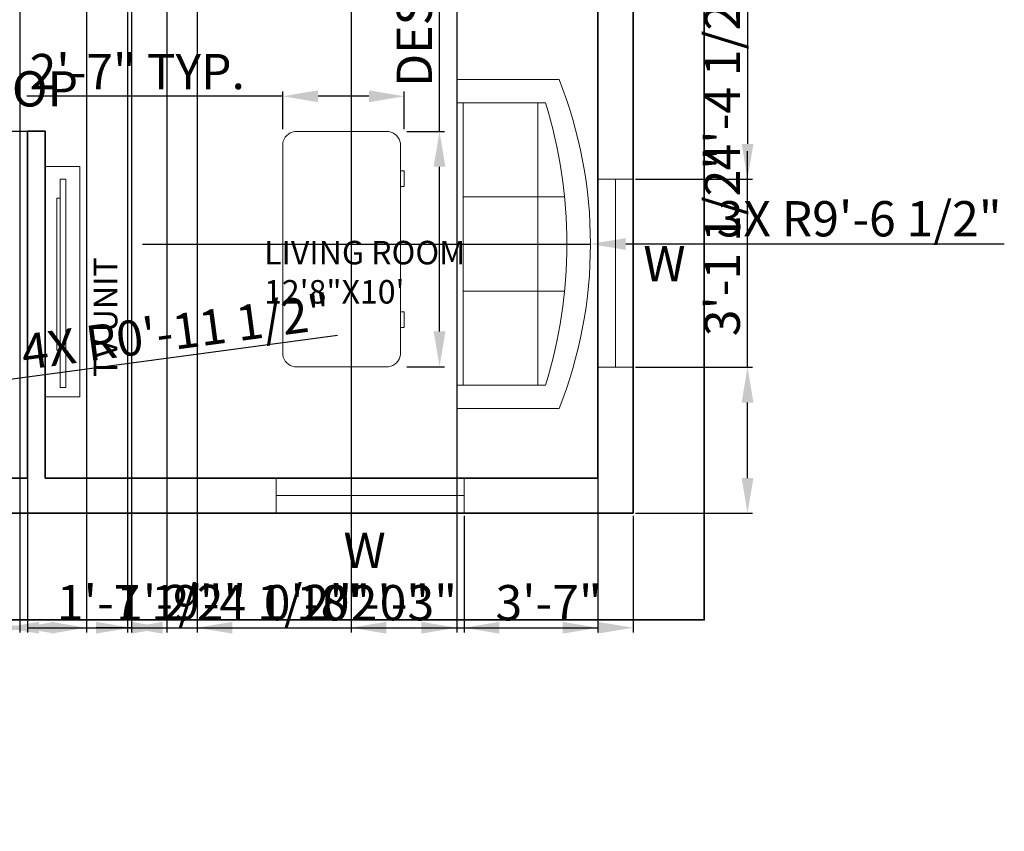
# Model space of a CAD drawing. Units: inches. Extents: x 53076 to 53578, y 41072 to 41816.
# Tile 2 of 4: x 53326 to 53578, y 41072 to 41279. Entities that reach past the tile are written whole.
import ezdxf

# ---------------------------------------------------------------- set-up
doc = ezdxf.new("R2010")
doc.units = ezdxf.units.IN
for name, color, linetype, lineweight in [('A-ANNO-DIMS', 2, 'Continuous', 18), ('A-ANNO-TEXT', 7, 'Continuous', 18), ('A-ANNO-TTLB', 7, 'Continuous', 35), ('A-AREA-IDEN', 7, 'Continuous', 18), ('A-DOOR', 3, 'Continuous', 25), ('A-EQPM', 8, 'Continuous', 18), ('A-FLOR-CASE', 9, 'Continuous', 18), ('A-FURN', 8, 'Continuous', 18), ('A-GLAZ', 4, 'Continuous', 18), ('A-WALL', 7, 'Continuous', 35)]:
    doc.layers.add(name, color=color, linetype=linetype, lineweight=lineweight)
doc.styles.get("Standard").update_dxf_attribs({"font": 'arial.ttf'})
doc.dimstyles.new('ISO-25', dxfattribs={"dimtxt": 9, "dimasz": 9, "dimexe": 1.25, "dimexo": 0.625, "dimtad": 1, "dimdec": 1, "dimrnd": 9, "dimlunit": 3, "dimtxsty": 'Standard', "dimcen": 2.5, "dimadec": 0, "dimazin": 0, "dimtfac": 1, "dimtdec": 1, "dimtmove": 0, "dimatfit": 3, "dimfxl": 1, "dimarcsym": 0})

# ---------------------------------------------------------------- blocks, each defined once
blk = doc.blocks.new('Sofa - Roundback 7 ft.')
for p, q in [((-12.00002, -32.4421), (-12.00003, -6.5971)), ((11.99997, -32.4421), (11.99998, -6.5971)), ((-36.000027, -34), (-36.000027, -11.4696)), ((35.99998, -34), (35.99998, -11.4696)), ((-35.999844, -13.3819), (35.9998, -13.3819)), ((-36.000027, -32.4421), (35.99998, -32.4421))]:
    blk.add_line(p, q)
for points in [[(-36.000027, -34), (-42.000027, -34), (-42.000027, -8)], [(41.99998, -8), (41.99998, -34), (35.99998, -34)]]:
    blk.add_lwpolyline(points)
for centre, radius, start, end in [((0, -114.25), 114.25, 68.43141, 111.5686), ((-0.00001, -127.1968), 121.1968, 72.72033, 107.2797)]:
    blk.add_arc(centre, radius, start, end)
blk = doc.blocks.new('Desk - 30 x 60 in.')
for p, q in [((-26.999995, 0), (26.999995, 0)), ((-29.999995, -27), (-29.999995, -3)), ((29.999995, -3), (29.999995, -27)), ((26.999995, -30), (-26.999995, -30)), ((-20.000005, -30), (-20.000005, -31)), ((-16.000005, -31), (-16.000005, -30)), ((15.999995, -31), (15.999995, -30)), ((19.999995, -30), (19.999995, -31)), ((-20.000005, -31), (-16.000005, -31)), ((19.999995, -31), (15.999995, -31))]:
    blk.add_line(p, q)
for centre, start, end in [((-26.499995, -3.5), 98.1301, 171.8699), ((26.499995, -3.5), 8.130102, 81.8699), ((-26.499995, -26.5), 188.1301, 261.8699), ((26.499995, -26.5), 278.1301, 351.8699)]:
    blk.add_arc(centre, 3.535534, start, end)
blk = doc.blocks.new('WIN-48IN')
for p, q in [((0, 48), (9, 48)), ((4.5, 48), (4.5, 0)), ((0, 0), (9, 0))]:
    blk.add_line(p, q)
blk = doc.blocks.new('*D28')
at = {"layer": 'A-ANNO-DIMS', "color": 0, "lineweight": -2, "transparency": 16777216}
for p, q in [((53433.43, 41250.06), (53433.43, 41352.45)), ((53425.06, 41250.06), (53434.68, 41250.06)), ((53433.43, 41199.06), (53433.43, 41241.06)), ((53425.06, 41190.06), (53434.68, 41190.06))]:
    blk.add_line(p, q, dxfattribs=at)
at = {"layer": 'A-ANNO-DIMS', "color": 0, "transparency": 16777216}
for points in [[(53431.93, 41241.06), (53434.93, 41241.06), (53433.43, 41250.06)], [(53431.93, 41199.06), (53434.93, 41199.06), (53433.43, 41190.06)]]:
    blk.add_solid(points, dxfattribs=at)
at = {"layer": 'Defpoints', "color": 0, "transparency": 16777216}
for p in [(53424.43, 41250.06), (53433.43, 41250.06), (53424.43, 41190.06)]:
    blk.add_point(p, dxfattribs=at)
at = {"layer": 'A-ANNO-DIMS', "color": 0, "transparency": 16777216, "insert": (53428.16, 41305.75), "char_height": 9, "attachment_point": 5, "rotation": 90}
blk.add_mtext('DESK 5\'-0" TYP.', dxfattribs=at)
blk = doc.blocks.new('*D29')
at = {"layer": 'A-ANNO-DIMS', "color": 0, "lineweight": -2, "transparency": 16777216}
for p, q in [((53393.43, 41250.68), (53393.43, 41260.31)), ((53424.43, 41250.68), (53424.43, 41260.31)), ((53393.43, 41259.06), (53328.17, 41259.06)), ((53415.43, 41259.06), (53402.43, 41259.06))]:
    blk.add_line(p, q, dxfattribs=at)
at = {"layer": 'A-ANNO-DIMS', "color": 0, "transparency": 16777216}
for points in [[(53402.43, 41260.56), (53402.43, 41257.56), (53393.43, 41259.06)], [(53415.43, 41260.56), (53415.43, 41257.56), (53424.43, 41259.06)]]:
    blk.add_solid(points, dxfattribs=at)
at = {"layer": 'Defpoints', "color": 0, "transparency": 16777216}
for p in [(53393.43, 41259.06), (53393.43, 41250.06), (53424.43, 41250.06)]:
    blk.add_point(p, dxfattribs=at)
at = {"layer": 'A-ANNO-DIMS', "color": 0, "transparency": 16777216, "insert": (53356.3, 41264.2), "char_height": 9, "attachment_point": 5}
blk.add_mtext('2\'-7" TYP.', dxfattribs=at)
blk = doc.blocks.new('*D30')
at = {"layer": 'A-ANNO-DIMS', "color": 0, "lineweight": -2, "transparency": 16777216}
for p, q in [((53312.97, 41194.48), (53318.55, 41194.48)), ((53317.3, 41185.48), (53317.3, 41170.44)), ((53312.97, 41161.44), (53318.55, 41161.44)), ((53317.3, 41161.44), (53317.3, 41071.52))]:
    blk.add_line(p, q, dxfattribs=at)
at = {"layer": 'A-ANNO-DIMS', "color": 0, "transparency": 16777216}
for points in [[(53315.8, 41185.48), (53318.8, 41185.48), (53317.3, 41194.48)], [(53315.8, 41170.44), (53318.8, 41170.44), (53317.3, 41161.44)]]:
    blk.add_solid(points, dxfattribs=at)
at = {"layer": 'Defpoints', "color": 0, "transparency": 16777216}
for p in [(53312.34, 41194.48), (53312.34, 41161.44), (53317.3, 41161.44)]:
    blk.add_point(p, dxfattribs=at)
at = {"layer": 'A-ANNO-DIMS', "color": 0, "transparency": 16777216, "insert": (53312.02, 41111.98), "char_height": 9, "attachment_point": 5, "rotation": 90}
blk.add_mtext('WC 2\'-9" TYP.', dxfattribs=at)
blk = doc.blocks.new('*D34')
at = {"layer": 'A-ANNO-DIMS', "color": 0, "lineweight": -2, "transparency": 16777216}
for p, q in [((53353.81, 41379.03), (53353.81, 41122.21)), ((53473.81, 41379.03), (53473.81, 41122.21)), ((53362.81, 41123.46), (53464.81, 41123.46))]:
    blk.add_line(p, q, dxfattribs=at)
at = {"layer": 'A-ANNO-DIMS', "color": 0, "transparency": 16777216}
for points in [[(53362.81, 41124.96), (53362.81, 41121.96), (53353.81, 41123.46)], [(53464.81, 41124.96), (53464.81, 41121.96), (53473.81, 41123.46)]]:
    blk.add_solid(points, dxfattribs=at)
at = {"layer": 'Defpoints', "color": 0, "transparency": 16777216}
for p in [(53353.81, 41379.66), (53473.81, 41379.66), (53473.81, 41123.46)]:
    blk.add_point(p, dxfattribs=at)
at = {"layer": 'A-ANNO-DIMS', "color": 0, "transparency": 16777216, "insert": (53413.81, 41128.68), "char_height": 9, "attachment_point": 5}
blk.add_mtext('10\'-0"', dxfattribs=at)
blk = doc.blocks.new('*D35')
at = {"layer": 'A-ANNO-DIMS', "color": 0, "lineweight": -2, "transparency": 16777216}
for p, q in [((53483.43, 41290.66), (53513.26, 41290.66)), ((53512.01, 41281.66), (53512.01, 41246.92)), ((53483.43, 41237.92), (53513.26, 41237.92))]:
    blk.add_line(p, q, dxfattribs=at)
at = {"layer": 'A-ANNO-DIMS', "color": 0, "transparency": 16777216}
for points in [[(53510.51, 41281.66), (53513.51, 41281.66), (53512.01, 41290.66)], [(53510.51, 41246.92), (53513.51, 41246.92), (53512.01, 41237.92)]]:
    blk.add_solid(points, dxfattribs=at)
at = {"layer": 'Defpoints', "color": 0, "transparency": 16777216}
for p in [(53482.81, 41290.66), (53482.81, 41237.92), (53512.01, 41237.92)]:
    blk.add_point(p, dxfattribs=at)
at = {"layer": 'A-ANNO-DIMS', "color": 0, "transparency": 16777216, "insert": (53506.73, 41264.29), "char_height": 9, "attachment_point": 5, "rotation": 90}
blk.add_mtext('4\'-4 1/2"', dxfattribs=at)
blk = doc.blocks.new('*D37')
at = {"layer": 'A-ANNO-DIMS', "color": 0, "lineweight": -2, "transparency": 16777216}
for p, q in [((53326.31, 41520.3), (53326.31, 41122.21)), ((53354.81, 41520.3), (53354.81, 41122.21)), ((53335.31, 41123.46), (53345.81, 41123.46)), ((53354.81, 41123.46), (53410.11, 41123.46))]:
    blk.add_line(p, q, dxfattribs=at)
at = {"layer": 'A-ANNO-DIMS', "color": 0, "transparency": 16777216}
for points in [[(53335.31, 41124.96), (53335.31, 41121.96), (53326.31, 41123.46)], [(53345.81, 41124.96), (53345.81, 41121.96), (53354.81, 41123.46)]]:
    blk.add_solid(points, dxfattribs=at)
at = {"layer": 'Defpoints', "color": 0, "transparency": 16777216}
for p in [(53326.31, 41520.92), (53354.81, 41520.92), (53354.81, 41123.46)]:
    blk.add_point(p, dxfattribs=at)
at = {"layer": 'A-ANNO-DIMS', "color": 0, "transparency": 16777216, "insert": (53386.96, 41128.73), "char_height": 9, "attachment_point": 5}
blk.add_mtext('2\'-4 1/2"', dxfattribs=at)
blk = doc.blocks.new('*D44')
at = {"layer": 'A-ANNO-DIMS', "color": 0, "lineweight": -2, "transparency": 16777216}
for p, q in [((53439.72, 41152.03), (53439.72, 41122.21)), ((53482.81, 41152.03), (53482.81, 41122.21)), ((53448.72, 41123.46), (53473.81, 41123.46))]:
    blk.add_line(p, q, dxfattribs=at)
at = {"layer": 'A-ANNO-DIMS', "color": 0, "transparency": 16777216}
for points in [[(53448.72, 41124.96), (53448.72, 41121.96), (53439.72, 41123.46)], [(53473.81, 41124.96), (53473.81, 41121.96), (53482.81, 41123.46)]]:
    blk.add_solid(points, dxfattribs=at)
at = {"layer": 'Defpoints', "color": 0, "transparency": 16777216}
for p in [(53439.72, 41152.66), (53482.81, 41152.66), (53482.81, 41123.46)]:
    blk.add_point(p, dxfattribs=at)
at = {"layer": 'A-ANNO-DIMS', "color": 0, "transparency": 16777216, "insert": (53461.27, 41128.68), "char_height": 9, "attachment_point": 5}
blk.add_mtext('3\'-7"', dxfattribs=at)
blk = doc.blocks.new('*D49')
at = {"layer": 'A-ANNO-DIMS', "color": 0, "lineweight": -2, "transparency": 16777216}
for p, q in [((53512.01, 41189.92), (53512.01, 41245.06)), ((53483.43, 41189.92), (53513.26, 41189.92)), ((53512.01, 41161.66), (53512.01, 41180.92)), ((53483.43, 41152.66), (53513.26, 41152.66))]:
    blk.add_line(p, q, dxfattribs=at)
at = {"layer": 'A-ANNO-DIMS', "color": 0, "transparency": 16777216}
for points in [[(53510.51, 41180.92), (53513.51, 41180.92), (53512.01, 41189.92)], [(53510.51, 41161.66), (53513.51, 41161.66), (53512.01, 41152.66)]]:
    blk.add_solid(points, dxfattribs=at)
at = {"layer": 'Defpoints', "color": 0, "transparency": 16777216}
for p in [(53482.81, 41189.92), (53512.01, 41189.92), (53482.81, 41152.66)]:
    blk.add_point(p, dxfattribs=at)
at = {"layer": 'A-ANNO-DIMS', "color": 0, "transparency": 16777216, "insert": (53506.72, 41221.99), "char_height": 9, "attachment_point": 5, "rotation": 90}
blk.add_mtext('3\'-1 1/2"', dxfattribs=at)
blk = doc.blocks.new('*D55')
at = {"layer": 'A-ANNO-DIMS', "color": 0, "lineweight": -2, "transparency": 16777216}
for p, q in [((53322.2, 41589.03), (53322.2, 41122.21)), ((53343.31, 41584.53), (53343.31, 41122.21)), ((53331.2, 41123.46), (53334.31, 41123.46)), ((53343.31, 41123.46), (53376.63, 41123.46))]:
    blk.add_line(p, q, dxfattribs=at)
at = {"layer": 'A-ANNO-DIMS', "color": 0, "transparency": 16777216}
for points in [[(53331.2, 41124.96), (53331.2, 41121.96), (53322.2, 41123.46)], [(53334.31, 41124.96), (53334.31, 41121.96), (53343.31, 41123.46)]]:
    blk.add_solid(points, dxfattribs=at)
at = {"layer": 'Defpoints', "color": 0, "transparency": 16777216}
for p in [(53322.2, 41589.66), (53343.31, 41585.16), (53343.31, 41123.46)]:
    blk.add_point(p, dxfattribs=at)
at = {"layer": 'A-ANNO-DIMS', "color": 0, "transparency": 16777216, "insert": (53364.47, 41128.68), "char_height": 9, "attachment_point": 5}
blk.add_mtext('1\'-9"', dxfattribs=at)
blk = doc.blocks.new('*D64')
at = {"layer": 'A-ANNO-DIMS', "color": 0, "lineweight": -2, "transparency": 16777216}
for p, q in [((53363.81, 41456.53), (53363.81, 41122.21)), ((53371.57, 41456.53), (53371.57, 41122.21)), ((53354.81, 41123.46), (53345.81, 41123.46)), ((53363.81, 41123.46), (53371.57, 41123.46)), ((53380.57, 41123.46), (53414.74, 41123.46))]:
    blk.add_line(p, q, dxfattribs=at)
at = {"layer": 'A-ANNO-DIMS', "color": 0, "transparency": 16777216}
for points in [[(53354.81, 41124.96), (53354.81, 41121.96), (53363.81, 41123.46)], [(53380.57, 41124.96), (53380.57, 41121.96), (53371.57, 41123.46)]]:
    blk.add_solid(points, dxfattribs=at)
at = {"layer": 'Defpoints', "color": 0, "transparency": 16777216}
for p in [(53363.81, 41457.16), (53371.57, 41457.16), (53371.57, 41123.46)]:
    blk.add_point(p, dxfattribs=at)
at = {"layer": 'A-ANNO-DIMS', "color": 0, "transparency": 16777216, "insert": (53402.15, 41128.68), "char_height": 9, "attachment_point": 5}
blk.add_mtext('0\'-8"', dxfattribs=at)
blk = doc.blocks.new('*D65')
at = {"layer": 'A-ANNO-DIMS', "color": 0, "lineweight": -2, "transparency": 16777216}
for p, q in [((53410.86, 41483.76), (53410.86, 41122.21)), ((53437.81, 41456.53), (53437.81, 41122.21)), ((53419.86, 41123.46), (53428.81, 41123.46))]:
    blk.add_line(p, q, dxfattribs=at)
at = {"layer": 'A-ANNO-DIMS', "color": 0, "transparency": 16777216}
for points in [[(53419.86, 41124.96), (53419.86, 41121.96), (53410.86, 41123.46)], [(53428.81, 41124.96), (53428.81, 41121.96), (53437.81, 41123.46)]]:
    blk.add_solid(points, dxfattribs=at)
at = {"layer": 'Defpoints', "color": 0, "transparency": 16777216}
for p in [(53410.86, 41484.39), (53437.81, 41457.16), (53437.81, 41123.46)]:
    blk.add_point(p, dxfattribs=at)
at = {"layer": 'A-ANNO-DIMS', "color": 0, "transparency": 16777216, "insert": (53424.33, 41128.68), "char_height": 9, "attachment_point": 5}
blk.add_mtext('2\'-3"', dxfattribs=at)
blk = doc.blocks.new('*D68')
at = {"layer": 'A-ANNO-DIMS', "color": 0, "lineweight": -2, "transparency": 16777216}
for p, q in [((53155.81, 41273.53), (53155.81, 41122.21)), ((53326.31, 41273.53), (53326.31, 41122.21)), ((53164.81, 41123.46), (53317.31, 41123.46))]:
    blk.add_line(p, q, dxfattribs=at)
at = {"layer": 'A-ANNO-DIMS', "color": 0, "transparency": 16777216}
for points in [[(53164.81, 41124.96), (53164.81, 41121.96), (53155.81, 41123.46)], [(53317.31, 41124.96), (53317.31, 41121.96), (53326.31, 41123.46)]]:
    blk.add_solid(points, dxfattribs=at)
at = {"layer": 'Defpoints', "color": 0, "transparency": 16777216}
for p in [(53155.81, 41274.16), (53326.31, 41274.16), (53326.31, 41123.46)]:
    blk.add_point(p, dxfattribs=at)
at = {"layer": 'A-ANNO-DIMS', "color": 0, "transparency": 16777216, "insert": (53241.06, 41128.73), "char_height": 9, "attachment_point": 5}
blk.add_mtext('14\'-2 1/2"', dxfattribs=at)
blk = doc.blocks.new('*D69')
at = {"layer": 'A-ANNO-DIMS', "color": 0, "lineweight": -2, "transparency": 16777216}
for p, q in [((53328.31, 41249.53), (53328.31, 41122.21)), ((53308.69, 41245.03), (53308.69, 41122.21)), ((53317.69, 41123.46), (53319.31, 41123.46)), ((53328.31, 41123.46), (53382.6, 41123.46))]:
    blk.add_line(p, q, dxfattribs=at)
at = {"layer": 'A-ANNO-DIMS', "color": 0, "transparency": 16777216}
for points in [[(53317.69, 41124.96), (53317.69, 41121.96), (53308.69, 41123.46)], [(53319.31, 41124.96), (53319.31, 41121.96), (53328.31, 41123.46)]]:
    blk.add_solid(points, dxfattribs=at)
at = {"layer": 'Defpoints', "color": 0, "transparency": 16777216}
for p in [(53328.31, 41250.16), (53308.69, 41245.66), (53328.31, 41123.46)]:
    blk.add_point(p, dxfattribs=at)
at = {"layer": 'A-ANNO-DIMS', "color": 0, "transparency": 16777216, "insert": (53359.96, 41128.73), "char_height": 9, "attachment_point": 5}
blk.add_mtext('1\'-7 1/2"', dxfattribs=at)
blk = doc.blocks.new('*D72')
at = {"layer": 'A-ANNO-DIMS', "color": 0, "lineweight": -2, "transparency": 16777216}
for p, q in [((53357.68, 41221.36), (53471.93, 41221.36)), ((53577.53, 41221.36), (53480.93, 41221.36))]:
    blk.add_line(p, q, dxfattribs=at)
at = {"layer": 'A-ANNO-DIMS', "color": 0, "transparency": 16777216}
blk.add_solid([(53480.93, 41222.86), (53480.93, 41219.86), (53471.93, 41221.36)], dxfattribs=at)
at = {"layer": 'Defpoints', "color": 0, "transparency": 16777216}
for p in [(53357.68, 41221.36), (53471.93, 41221.36)]:
    blk.add_point(p, dxfattribs=at)
at = {"layer": 'A-ANNO-DIMS', "color": 0, "transparency": 16777216, "insert": (53540.48, 41226.64), "char_height": 9, "attachment_point": 5, "rotation": 0.0002}
blk.add_mtext('3X R9\'-6 1/2"', dxfattribs=at)
blk = doc.blocks.new('*D74')
at = {"layer": 'A-ANNO-DIMS', "color": 0, "lineweight": -2, "transparency": 16777216}
for p, q in [((53407.43, 41198.01), (53317.79, 41185.96)), ((53297.64, 41183.25), (53308.87, 41184.76))]:
    blk.add_line(p, q, dxfattribs=at)
at = {"layer": 'A-ANNO-DIMS', "color": 0, "transparency": 16777216}
blk.add_solid([(53317.59, 41187.45), (53317.99, 41184.48), (53308.87, 41184.76)], dxfattribs=at)
at = {"layer": 'Defpoints', "color": 0, "transparency": 16777216}
for p in [(53297.64, 41183.25), (53308.87, 41184.76)]:
    blk.add_point(p, dxfattribs=at)
at = {"layer": 'A-ANNO-DIMS', "color": 0, "transparency": 16777216, "insert": (53366.37, 41197.82), "char_height": 9, "attachment_point": 5, "rotation": 7.6564}
blk.add_mtext('4X R0\'-11 1/2"', dxfattribs=at)

msp = doc.modelspace()

# ---------------------------------------------------------------- linework, layer by layer
at = {"layer": 'A-ANNO-TTLB'}
msp.add_lwpolyline([(53105.85, 41713.9), (53500.98, 41713.9), (53500.98, 41125.46), (53105.85, 41125.46)], close=True, dxfattribs=at)
at = {"layer": 'A-DOOR'}
msp.add_line((53308.69, 41250.16), (53328.31, 41250.16), dxfattribs=at)
at = {"layer": 'A-EQPM'}
for p, q in [((53336.67, 41233.05), (53335.77, 41233.05)), ((53335.77, 41233.05), (53335.77, 41194.31)), ((53335.77, 41194.31), (53336.67, 41194.31))]:
    msp.add_line(p, q, dxfattribs=at)
msp.add_lwpolyline([(53336.67, 41237.93), (53338.04, 41237.93), (53338.04, 41184.76), (53336.67, 41184.76)], close=True, dxfattribs=at)
at = {"layer": 'A-FLOR-CASE'}
for p, q in [((53332.81, 41241.11), (53332.81, 41241.11)), ((53332.81, 41241.11), (53341.67, 41241.11)), ((53341.67, 41241.11), (53341.67, 41182.35)), ((53341.67, 41182.35), (53332.81, 41182.35))]:
    msp.add_line(p, q, dxfattribs=at)
at = {"layer": 'A-WALL'}
for p, q in [((53482.81, 41290.66), (53482.81, 41152.66)), ((53473.81, 41281.66), (53473.81, 41161.66)), ((53328.31, 41161.66), (53328.31, 41250.16)), ((53332.81, 41250.16), (53328.31, 41250.16)), ((53332.81, 41161.66), (53332.81, 41250.16)), ((53328.31, 41161.66), (53280.31, 41161.66)), ((53473.81, 41161.66), (53332.81, 41161.66)), ((53482.81, 41152.66), (53146.81, 41152.66))]:
    msp.add_line(p, q, dxfattribs=at)

# ---------------------------------------------------------------- block references
at = {"layer": 'A-FURN'}
for name, p, rotation in [('Sofa - Roundback 7 ft.', (53471.93, 41221.36), 269.9999999999999), ('Desk - 30 x 60 in.', (53393.43, 41220.06), 89.9999999999713)]:
    msp.add_blockref(name, p, dxfattribs=dict(at, rotation=rotation))
at = {"layer": 'A-GLAZ'}
msp.add_blockref('WIN-48IN', (53473.81, 41189.92), dxfattribs=at)
at = {"layer": 'A-GLAZ', "rotation": 270}
msp.add_blockref('WIN-48IN', (53391.72, 41161.66), dxfattribs=at)

# ---------------------------------------------------------------- texts
at = {"layer": 'A-ANNO-TEXT', "char_height": 9, "attachment_point": 1}
for s, insert in [('OP ', (53324.32, 41265.45)), ('W ', (53485.43, 41220.88)), ('W ', (53408.92, 41147.71))]:
    msp.add_mtext_dynamic_manual_height_columns(s, width=6.4326, gutter_width=12.5, heights=[0], dxfattribs=dict(at, insert=insert))
at = {"layer": 'A-ANNO-TEXT', "insert": (53345.22, 41187.41), "char_height": 6, "attachment_point": 1, "rotation": 90}
msp.add_mtext_dynamic_manual_height_columns('TV UNIT', width=85.6025, gutter_width=12.5, heights=[0], dxfattribs=at)
at = {"layer": 'A-AREA-IDEN', "insert": (53388.65, 41222.17), "char_height": 6, "attachment_point": 1}
msp.add_mtext_dynamic_manual_height_columns('LIVING ROOM\\P12\'8"X10\'', width=85.6025, gutter_width=12.5, heights=[0], dxfattribs=at)

# ---------------------------------------------------------------- dimensions: what is measured, and where the dimension line sits
at = {"layer": 'A-ANNO-DIMS'}
for base, p1, p2, picture, middle in [((53343.31, 41123.46), (53322.2, 41589.66), (53343.31, 41585.16), '*D55', (53364.47, 41128.68)), ((53354.81, 41123.46), (53326.31, 41520.92), (53354.81, 41520.92), '*D37', (53386.96, 41128.73)), ((53437.8064, 41123.456), (53410.8553, 41484.3893), (53437.8064, 41457.156), '*D65', (53424.3308, 41128.6792)), ((53371.57, 41123.46), (53363.81, 41457.16), (53371.57, 41457.16), '*D64', (53402.15, 41128.68)), ((53473.81, 41123.46), (53353.81, 41379.66), (53473.81, 41379.66), '*D34', (53413.81, 41128.68)), ((53326.31, 41123.46), (53155.81, 41274.16), (53326.31, 41274.16), '*D68', (53241.06, 41128.73)), ((53328.31, 41123.46), (53308.69, 41245.66), (53328.31, 41250.16), '*D69', (53359.96, 41128.73)), ((53482.81, 41123.46), (53439.72, 41152.66), (53482.81, 41152.66), '*D44', (53461.27, 41128.68))]:
    dim = msp.add_linear_dim(base=base, p1=p1, p2=p2, dimstyle='ISO-25', override={"dimdec": 1, "dimlfac": 1, "dimrnd": 0, "dimzin": 1, "dimdsep": 46, "dimlunit": 4, "dimfrac": 2}, dxfattribs=at)
    dim.commit()
    dim.dimension.update_dxf_attribs({"geometry": picture, "text_midpoint": middle})
for base, p1, p2, angle, text, picture, middle in [((53433.43, 41250.06), (53424.43, 41190.06), (53424.43, 41250.06), 90, 'DESK <> TYP.', '*D28', (53428.16, 41305.75)), ((53393.43, 41259.06), (53424.43, 41250.06), (53393.43, 41250.06), 180, '<> TYP.', '*D29', (53356.3, 41264.2)), ((53317.3, 41161.44), (53312.34, 41194.48), (53312.34, 41161.44), 270, 'WC <> TYP.', '*D30', (53312.02, 41111.98))]:
    dim = msp.add_linear_dim(base=base, p1=p1, p2=p2, angle=angle, text=text, dimstyle='ISO-25', override={"dimdec": 1, "dimlfac": 1, "dimrnd": 0, "dimzin": 1, "dimdsep": 46, "dimlunit": 4, "dimfrac": 2}, dxfattribs=at)
    dim.commit()
    dim.dimension.update_dxf_attribs({"geometry": picture, "text_midpoint": middle})
for base, p1, p2, picture, middle in [((53512.01, 41237.92), (53482.81, 41290.66), (53482.81, 41237.92), '*D35', (53506.73, 41264.29)), ((53512.01, 41189.92), (53482.81, 41152.66), (53482.81, 41189.92), '*D49', (53506.72, 41221.99))]:
    dim = msp.add_linear_dim(base=base, p1=p1, p2=p2, angle=90, dimstyle='ISO-25', override={"dimdec": 1, "dimlfac": 1, "dimrnd": 0, "dimzin": 1, "dimdsep": 46, "dimlunit": 4, "dimfrac": 2}, dxfattribs=at)
    dim.commit()
    dim.dimension.update_dxf_attribs({"geometry": picture, "text_midpoint": middle})
dim = msp.add_radius_dim(center=(53357.68006, 41221.357667), mpoint=(53471.93006, 41221.358), text='3X <>', dimstyle='ISO-25', override={"dimdec": 1, "dimlfac": 1, "dimrnd": 0, "dimzin": 1, "dimdsep": 46, "dimlunit": 4, "dimfrac": 2}, dxfattribs=at)
dim.commit()
dim.dimension.update_dxf_attribs({"geometry": '*D72', "text_midpoint": (53540.48006, 41221.3581998), "dimtype": 164})
dim = msp.add_radius_dim(center=(53297.64, 41183.25), mpoint=(53308.87, 41184.76), text='4X <>', dimstyle='ISO-25', override={"dimdec": 1, "dimlfac": 1, "dimrnd": 0, "dimzin": 1, "dimdsep": 46, "dimlunit": 4, "dimfrac": 2}, dxfattribs=at)
dim.commit()
dim.dimension.update_dxf_attribs({"geometry": '*D74', "text_midpoint": (53366.37, 41197.82)})

doc.saveas('drawing.dxf')
